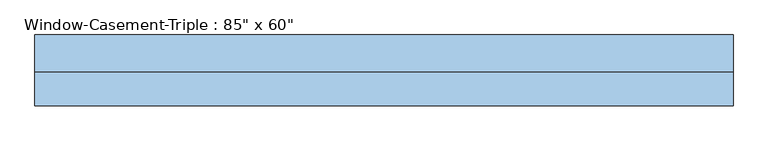
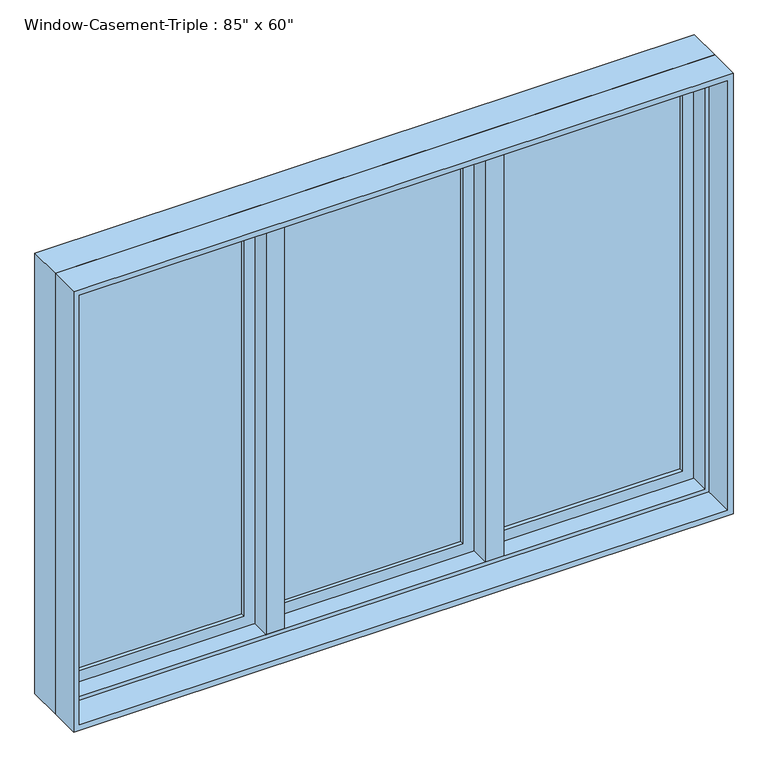
"""IFC4 building model written with IfcOpenShell, lengths in millimetres: window geometry."""

from ifc_helpers import new_model, si_unit, frame, origin, place, context, project, spatial, polyline, outline, extrude, faceted_brep, source, transform, mapped, element, save


def window_45599283(model_context):
    return source(origin(), model_context, "Body", "SolidModel", [
        faceted_brep([(1047.75, 68.25, 2406.65), (1047.75, 4.75, 2406.65), (-1047.75, 4.75, 2406.65), (-1047.75, 68.25, 2406.65), (1066.8, 119.05, 2425.7), (1066.8, 68.25, 2425.7), (-1066.8, 68.25, 2425.7), (-1066.8, 119.05, 2425.7), (1079.5, 4.75, 2438.4), (1079.5, 119.05, 2438.4), (-1079.5, 119.05, 2438.4), (-1079.5, 4.75, 2438.4), (-1047.75, 4.75, 946.15), (-1047.75, 68.25, 946.15), (-1066.8, 68.25, 927.1), (-1066.8, 119.05, 927.1), (-1079.5, 119.05, 914.4), (-1079.5, 4.75, 914.4), (1047.75, 4.75, 946.15), (1047.75, 68.25, 946.15), (1066.8, 68.25, 927.1), (1066.8, 119.05, 927.1), (1079.5, 119.05, 914.4), (1079.5, 4.75, 914.4)], [[[0, 1, 2, 3]], [[4, 5, 6, 7]], [[8, 9, 10, 11]], [[3, 2, 12, 13]], [[7, 6, 14, 15]], [[11, 10, 16, 17]], [[13, 12, 18, 19]], [[15, 14, 20, 21]], [[17, 16, 22, 23]], [[11, 17, 23, 8], [1, 18, 12, 2]], [[19, 18, 1, 0]], [[5, 20, 14, 6], [3, 13, 19, 0]], [[21, 20, 5, 4]], [[23, 22, 9, 8]], [[9, 22, 16, 10], [7, 15, 21, 4]]]),
        extrude(outline(polyline([(2438.4, -1079.5), (914.4, -1079.5), (914.4, 1079.5), (2438.4, 1079.5), (2438.4, -1079.5)]), holes=[polyline([(2419.35, 1060.45), (933.45, 1060.45), (933.45, -1060.45), (2419.35, -1060.45), (2419.35, 1060.45)])]), frame((0.0, -100.0, 0.0), z_axis=(0.0, 1.0, 0.0), x_axis=(0.0, 0.0, 1.0)), (0.0, 0.0, 1.0), 104.75),
        extrude(outline(polyline([(927.1, 1066.8), (2425.7, 1066.8), (2425.7, 368.3), (927.1, 368.3), (927.1, 1066.8)]), holes=[polyline([(984.25, 425.45), (2368.55, 425.45), (2368.55, 1009.65), (984.25, 1009.65), (984.25, 425.45)])]), frame((0.0, 68.25, 0.0), z_axis=(0.0, 1.0, 0.0), x_axis=(0.0, 0.0, 1.0)), (0.0, 0.0, 1.0), 44.45),
        extrude(outline(polyline([(2425.7, -1066.8), (927.1, -1066.8), (927.1, -368.3), (2425.7, -368.3), (2425.7, -1066.8)]), holes=[polyline([(2368.55, -425.45), (984.25, -425.45), (984.25, -1009.65), (2368.55, -1009.65), (2368.55, -425.45)])]), frame((0.0, 68.25, 0.0), z_axis=(0.0, 1.0, 0.0), x_axis=(0.0, 0.0, 1.0)), (0.0, 0.0, 1.0), 44.45),
        extrude(outline(polyline([(1009.65, 100.0), (1009.65, 93.65), (425.45, 93.65), (425.45, 100.0), (1009.65, 100.0)])), frame((0.0, 0.0, 984.25), z_axis=(0.0, 0.0, 1.0), x_axis=(1.0, 0.0, 0.0)), (0.0, 0.0, 1.0), 1384.3),
        extrude(outline(polyline([(425.45, 80.95), (425.45, 87.3), (1009.65, 87.3), (1009.65, 80.95), (425.45, 80.95)])), frame((0.0, 0.0, 984.25), z_axis=(0.0, 0.0, 1.0), x_axis=(1.0, 0.0, 0.0)), (0.0, 0.0, 1.0), 1384.3),
        extrude(outline(polyline([(-425.45, 100.0), (-425.45, 93.65), (-1009.65, 93.65), (-1009.65, 100.0), (-425.45, 100.0)])), frame((0.0, 0.0, 984.25), z_axis=(0.0, 0.0, 1.0), x_axis=(1.0, 0.0, 0.0)), (0.0, 0.0, 1.0), 1384.3),
        extrude(outline(polyline([(-1009.65, 80.95), (-1009.65, 87.3), (-425.45, 87.3), (-425.45, 80.95), (-1009.65, 80.95)])), frame((0.0, 0.0, 984.25), z_axis=(0.0, 0.0, 1.0), x_axis=(1.0, 0.0, 0.0)), (0.0, 0.0, 1.0), 1384.3),
        extrude(outline(polyline([(292.1, 100.0), (292.1, 93.65), (-292.1, 93.65), (-292.1, 100.0), (292.1, 100.0)])), frame((0.0, 0.0, 984.25), z_axis=(0.0, 0.0, 1.0), x_axis=(1.0, 0.0, 0.0)), (0.0, 0.0, 1.0), 1384.3),
        extrude(outline(polyline([(-292.1, 80.95), (-292.1, 87.3), (292.1, 87.3), (292.1, 80.95), (-292.1, 80.95)])), frame((0.0, 0.0, 984.25), z_axis=(0.0, 0.0, 1.0), x_axis=(1.0, 0.0, 0.0)), (0.0, 0.0, 1.0), 1384.3),
        extrude(outline(polyline([(927.1, 349.25), (2425.7, 349.25), (2425.7, -349.25), (927.1, -349.25), (927.1, 349.25)]), holes=[polyline([(984.25, -292.1), (2368.55, -292.1), (2368.55, 292.1), (984.25, 292.1), (984.25, -292.1)])]), frame((0.0, 68.25, 0.0), z_axis=(0.0, 1.0, 0.0), x_axis=(0.0, 0.0, 1.0)), (0.0, 0.0, 1.0), 44.45),
        faceted_brep([(-368.3, 68.25, 2425.7), (-388.8101338, 68.25, 2425.7), (-388.8101338, 4.75, 2425.7), (-328.7398662, 4.75, 2425.7), (-328.7398662, 68.25, 2425.7), (-349.25, 68.25, 2425.7), (-349.25, 119.05, 2425.7), (-368.3, 119.05, 2425.7), (-368.3, 119.05, 927.1), (-349.25, 119.05, 927.1), (-349.25, 90.475, 927.1), (-368.3, 90.475, 927.1), (-388.8101338, 68.25, 2419.35), (-388.8101338, 4.75, 2419.35), (-388.8101338, 68.25, 2406.65), (-388.8101338, 68.25, 946.15), (-388.8101338, 4.75, 946.15), (-388.8101338, 4.75, 2406.65), (-328.7398662, 4.75, 2419.35), (-328.7398662, 4.75, 946.15), (-328.7398662, 4.75, 2406.65), (-328.7398662, 68.25, 2419.35), (-328.7398662, 68.25, 946.15), (-328.7398662, 68.25, 2406.65), (-349.25, 68.25, 2419.35), (-349.25, 90.475, 2419.35), (-349.25, 90.475, 2406.65), (-349.25, 68.25, 2406.65), (-349.25, 68.25, 946.15), (-349.25, 90.475, 946.15), (-368.3, 90.475, 946.15), (-368.3, 68.25, 946.15), (-368.3, 68.25, 2406.65), (-368.3, 90.475, 2406.65), (-368.3, 90.475, 2419.35), (-368.3, 68.25, 2419.35)], [[[0, 1, 2, 3, 4, 5, 6, 7]], [[8, 9, 10, 11]], [[2, 1, 12, 13]], [[14, 15, 16, 17]], [[3, 2, 13, 18]], [[17, 16, 19, 20]], [[4, 3, 18, 21]], [[20, 19, 22, 23]], [[6, 5, 24, 25, 26, 27, 28, 29, 10, 9]], [[0, 7, 8, 11, 30, 31, 32, 33, 34, 35]], [[25, 34, 33, 26]], [[29, 30, 11, 10]], [[34, 25, 24, 21, 18, 13, 12, 35]], [[26, 33, 32, 14, 17, 20, 23, 27]], [[30, 29, 28, 22, 19, 16, 15, 31]], [[1, 0, 35, 12]], [[15, 14, 32, 31]], [[5, 4, 21, 24]], [[28, 27, 23, 22]], [[7, 6, 9, 8]]]),
        faceted_brep([(349.25, 68.25, 2425.7), (328.7398662, 68.25, 2425.7), (328.7398662, 4.75, 2425.7), (388.8101338, 4.75, 2425.7), (388.8101338, 68.25, 2425.7), (368.3, 68.25, 2425.7), (368.3, 119.05, 2425.7), (349.25, 119.05, 2425.7), (349.25, 119.05, 927.1), (368.3, 119.05, 927.1), (368.3, 90.475, 927.1), (349.25, 90.475, 927.1), (328.7398662, 68.25, 2419.35), (328.7398662, 4.75, 2419.35), (328.7398662, 68.25, 2406.65), (328.7398662, 68.25, 946.15), (328.7398662, 4.75, 946.15), (328.7398662, 4.75, 2406.65), (388.8101338, 4.75, 2419.35), (388.8101338, 4.75, 946.15), (388.8101338, 4.75, 2406.65), (388.8101338, 68.25, 2419.35), (388.8101338, 68.25, 946.15), (388.8101338, 68.25, 2406.65), (368.3, 68.25, 2419.35), (368.3, 90.475, 2419.35), (368.3, 90.475, 2406.65), (368.3, 68.25, 2406.65), (368.3, 68.25, 946.15), (368.3, 90.475, 946.15), (349.25, 90.475, 946.15), (349.25, 68.25, 946.15), (349.25, 68.25, 2406.65), (349.25, 90.475, 2406.65), (349.25, 90.475, 2419.35), (349.25, 68.25, 2419.35)], [[[0, 1, 2, 3, 4, 5, 6, 7]], [[8, 9, 10, 11]], [[2, 1, 12, 13]], [[14, 15, 16, 17]], [[3, 2, 13, 18]], [[17, 16, 19, 20]], [[4, 3, 18, 21]], [[20, 19, 22, 23]], [[6, 5, 24, 25, 26, 27, 28, 29, 10, 9]], [[0, 7, 8, 11, 30, 31, 32, 33, 34, 35]], [[25, 34, 33, 26]], [[29, 30, 11, 10]], [[34, 25, 24, 21, 18, 13, 12, 35]], [[26, 33, 32, 14, 17, 20, 23, 27]], [[30, 29, 28, 22, 19, 16, 15, 31]], [[1, 0, 35, 12]], [[15, 14, 32, 31]], [[5, 4, 21, 24]], [[28, 27, 23, 22]], [[7, 6, 9, 8]]]),
    ])


if __name__ == "__main__":
    model = new_model("IFC4")
    model_context = context("Model", 3, world=origin())
    ifc_project = project(units=[si_unit("LENGTHUNIT", "METRE", prefix="MILLI")], contexts=[model_context])
    site = spatial("IfcSite", under=ifc_project)
    building = spatial("IfcBuilding", under=site)
    placement = place(None, origin())
    window_shape = window_45599283(model_context)
    element("IfcWindow", 1, ObjectType="Window-Casement-Triple : 85\" x 60\"", at=placement, inside=building, context=model_context, shape_type="MappedRepresentation", body=[
        mapped(window_shape, transform((0.0, 0.0, 0.0), x_axis=(1.0, 0.0, 0.0), y_axis=(0.0, 1.0, 0.0), z_axis=(0.0, 0.0, 1.0))),
    ])
    save(model, "model.ifc")

# Revit data of these elements
# Type "Window-Casement-Triple : 85\" x 60\""
#   Type Mark = "18"
#   Fire Rating = "0.5h"
#   Assembly Code = "B2020100"
#   Analytic Construction = "Double glazing - domestic"
#   Window Inset [instance default] = 0' - 0"
#   Wall Thickness [instance default] = 0' - 6"
#   Muntin Width = 1' - 11"
#   Visual Light Transmittance = 0.81
#   Thermal Resistance (R) = 1.8146 (h·ft²·°F)/BTU
#   Solar Heat Gain Coefficient = 0.76
#   One Third Width = 2' - 4.33333"
#   Sash Width = 2' - 3 1/2"
#   Rough Width = 7' - 1 1/2"
#   Rough Height = 5' - 0 1/2"
#   Interior Wall Closure [instance default] = 0' - 2 1/4"
#   Height = 5' - 0"
#   Heat Transfer Coefficient (U) = 0.5511 BTU/(h·ft²·°F)
#   Muntin Height = 4' - 6 1/2"
#   Frame Extension [instance default] = 0' - 0 1/4"
#   Exterior Wall Closure [instance default] = 0' - 1 1/4"
#   Extension Jamb [instance default] = 0' - 2 1/4"
#   Default Sill Height = 3' - 0"
#   Width = 7' - 1"
#   Middle Muntin Visibility = yes
#   Side Muntin Visibility = yes
#   Interior Trim Visibility [instance default] = yes
#   Exterior Trim Visibility [instance default] = yes
#   Extension Jamb Visibility [instance default] = yes
#   Muntin Pattern = Muntin Pattern_2x2 : Muntin Pattern_2x2
#   Interior Trim Material = Wood - Stained
#   Interior Trim = Trim-Window-Interior-Flat : Picture Frame
#   Interior Frame Material = Wood - Stained
#   Glass Panel Material = Glass
#   Exterior Trim Material = Clad - White
#   Exterior Trim = Trim-Window-Exterior-Flat : with Sill
#   Exterior Frame Material = Clad - White
#   Wall Closure = (empty or 0)
# Element 1 (IfcWindow, "Window-Casement-Triple : 85\" x 60\"")
#   Wall Thickness = 0' - 7.87402"
#   Extension Jamb = 0' - 4.12402"
#   Materials on its faces: "Wood - Stained", "Glass", "Clad - White"
# Materials
#   "Wood - Stained": class "Wood", colour RGB 224 178 126, transparency 0, Cost = 0
#   "Glass": class "Glass", colour RGB 0 128 192, transparency 0.75, Description = "Soda Lime Glass", Cost = 0
#   "Clad - White": class "Wood", colour RGB 242 242 238, transparency 0, Cost = 0
